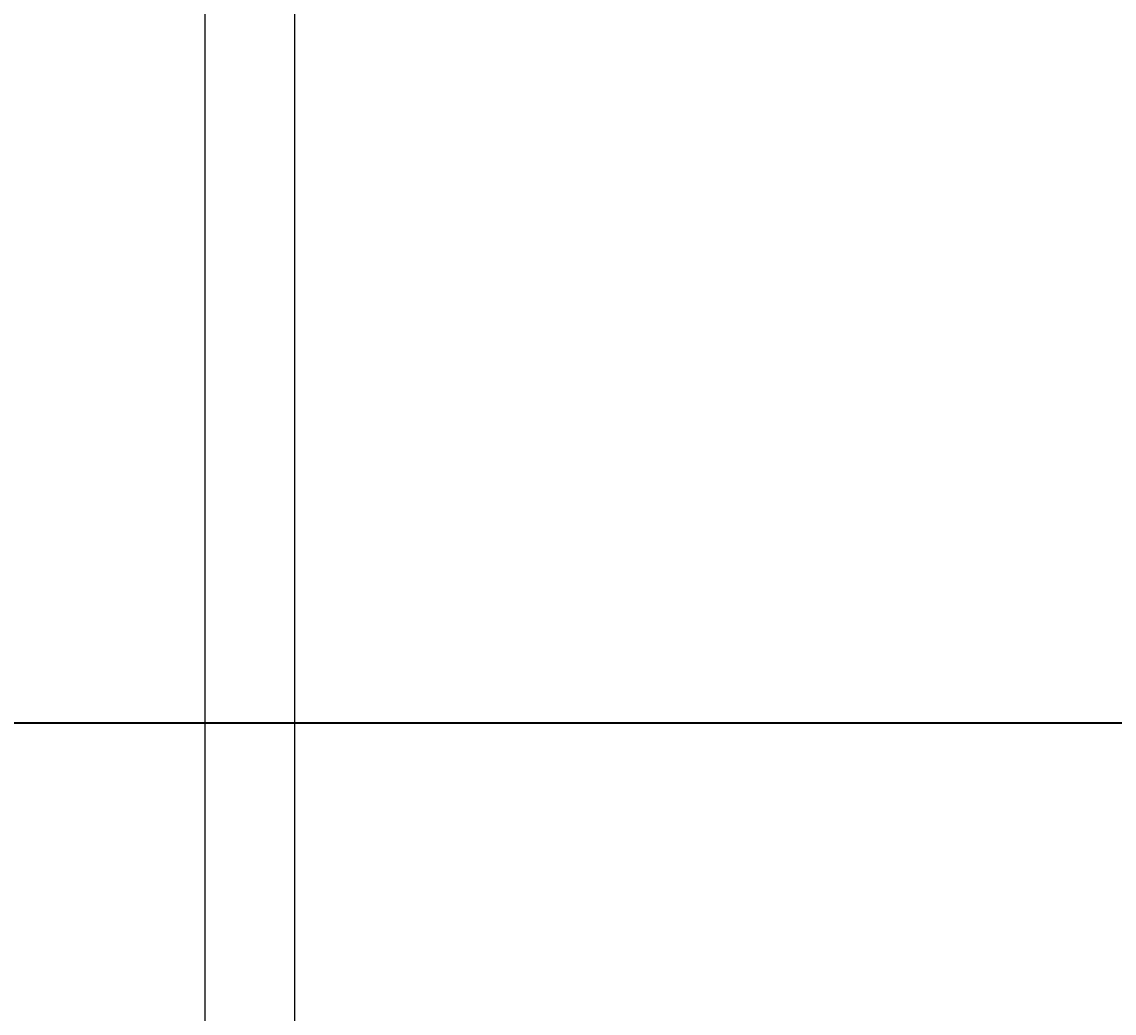
# Model space of a CAD drawing. Units: inches. Extents: x -6 to 289, y -8 to 323.
# Tile 94 of 107: x 196 to 222, y 252 to 276. Entities that reach past the tile are written whole.
import ezdxf

# ---------------------------------------------------------------- set-up
doc = ezdxf.new("R2010")
doc.units = ezdxf.units.IN
doc.header["$MEASUREMENT"] = 0
doc.layers.add('A-ANNO-DIMS', color=2, linetype='Continuous', lineweight=18)
doc.layers.add('A-ELEV', color=7, linetype='Continuous', lineweight=35)
doc.styles.get("Standard").update_dxf_attribs({"font": 'arial.ttf'})
doc.dimstyles.get("Standard").update_dxf_attribs({"dimtxt": 0.18, "dimasz": 0.18, "dimexe": 0.18, "dimexo": 0.0625, "dimgap": 0.09, "dimtad": 0, "dimtih": 1, "dimtoh": 1, "dimdec": 4, "dimzin": 0, "dimdsep": 46, "dimtxsty": 'Standard', "dimcen": 0.09, "dimadec": 0, "dimazin": 0, "dimtfac": 1, "dimtdec": 4, "dimtofl": 0, "dimtmove": 0, "dimatfit": 3, "dimfxl": 1, "dimtolj": 1, "dimtzin": 0, "dimarcsym": 0})

# ---------------------------------------------------------------- blocks, each defined once
blk = doc.blocks.new('*D13')
at = {"layer": 'A-ANNO-DIMS', "color": 0, "lineweight": -2, "transparency": 16777216}
for p, q in [((188.292, 226.951), (188.292, 322.969)), ((236.292, 226.951), (236.292, 322.969)), ((188.472, 322.789), (212.069, 322.789)), ((236.112, 322.789), (212.515, 322.789))]:
    blk.add_line(p, q, dxfattribs=at)
at = {"layer": 'A-ANNO-DIMS', "color": 0, "transparency": 16777216}
for points in [[(188.472, 322.819), (188.472, 322.759), (188.292, 322.789)], [(236.112, 322.819), (236.112, 322.759), (236.292, 322.789)]]:
    blk.add_solid(points, dxfattribs=at)
at = {"layer": 'Defpoints', "color": 0, "transparency": 16777216}
for p in [(236.292, 322.789), (188.292, 226.889), (236.292, 226.889)]:
    blk.add_point(p, dxfattribs=at)
at = {"layer": 'A-ANNO-DIMS', "color": 0, "transparency": 16777216, "insert": (212.292, 322.789), "char_height": 0.18, "attachment_point": 5}
blk.add_mtext('\\A1;48', dxfattribs=at)
blk = doc.blocks.new('*D27')
at = {"layer": 'A-ANNO-DIMS', "color": 0, "lineweight": -2, "transparency": 16777216}
for p, q in [((19.226, 307.289), (288.653, 307.289)), ((288.473, 307.109), (288.473, 277.471)), ((288.473, 247.469), (288.473, 277.107)), ((247.226, 247.289), (288.653, 247.289))]:
    blk.add_line(p, q, dxfattribs=at)
at = {"layer": 'A-ANNO-DIMS', "color": 0, "transparency": 16777216}
for points in [[(288.443, 307.109), (288.503, 307.109), (288.473, 307.289)], [(288.443, 247.469), (288.503, 247.469), (288.473, 247.289)]]:
    blk.add_solid(points, dxfattribs=at)
at = {"layer": 'Defpoints', "color": 0, "transparency": 16777216}
for p in [(19.164, 307.289), (288.473, 307.289), (247.164, 247.289)]:
    blk.add_point(p, dxfattribs=at)
at = {"layer": 'A-ANNO-DIMS', "color": 0, "transparency": 16777216, "insert": (288.473, 277.289), "char_height": 0.18, "attachment_point": 5}
blk.add_mtext('\\A1;60', dxfattribs=at)
blk = doc.blocks.new('*D80')
at = {"layer": 'A-ANNO-DIMS', "color": 0, "lineweight": -2, "transparency": 16777216}
for p, q in [((188.292, 116.842), (188.292, 322.969)), ((230.292, 116.842), (230.292, 322.969)), ((188.472, 322.789), (209.07, 322.789)), ((230.112, 322.789), (209.513, 322.789))]:
    blk.add_line(p, q, dxfattribs=at)
at = {"layer": 'A-ANNO-DIMS', "color": 0, "transparency": 16777216}
for points in [[(188.472, 322.819), (188.472, 322.759), (188.292, 322.789)], [(230.112, 322.819), (230.112, 322.759), (230.292, 322.789)]]:
    blk.add_solid(points, dxfattribs=at)
at = {"layer": 'Defpoints', "color": 0, "transparency": 16777216}
for p in [(230.292, 322.789), (188.292, 116.779), (230.292, 116.779)]:
    blk.add_point(p, dxfattribs=at)
at = {"layer": 'A-ANNO-DIMS', "color": 0, "transparency": 16777216, "insert": (209.292, 322.789), "char_height": 0.18, "attachment_point": 5}
blk.add_mtext('\\A1;42', dxfattribs=at)
blk = doc.blocks.new('*D96')
at = {"layer": 'A-ANNO-DIMS', "color": 0, "lineweight": -2, "transparency": 16777216}
for p, q in [((164.004, 159.411), (164.004, 322.969)), ((200.616, 159.411), (200.616, 322.969)), ((164.184, 322.789), (181.934, 322.789)), ((200.436, 322.789), (182.686, 322.789))]:
    blk.add_line(p, q, dxfattribs=at)
at = {"layer": 'A-ANNO-DIMS', "color": 0, "transparency": 16777216}
for points in [[(164.184, 322.819), (164.184, 322.759), (164.004, 322.789)], [(200.436, 322.819), (200.436, 322.759), (200.616, 322.789)]]:
    blk.add_solid(points, dxfattribs=at)
at = {"layer": 'Defpoints', "color": 0, "transparency": 16777216}
for p in [(200.616, 322.789), (164.004, 159.348), (200.616, 159.348)]:
    blk.add_point(p, dxfattribs=at)
at = {"layer": 'A-ANNO-DIMS', "color": 0, "transparency": 16777216, "insert": (182.31, 322.789), "char_height": 0.18, "attachment_point": 5}
blk.add_mtext('\\A1;36.61', dxfattribs=at)
blk = doc.blocks.new('*D97')
at = {"layer": 'A-ANNO-DIMS', "color": 0, "lineweight": -2, "transparency": 16777216}
for p, q in [((200.616, 159.411), (200.616, 322.969)), ((202.741, 159.411), (202.741, 322.969)), ((200.796, 322.789), (201.283, 322.789)), ((202.561, 322.789), (202.075, 322.789))]:
    blk.add_line(p, q, dxfattribs=at)
at = {"layer": 'A-ANNO-DIMS', "color": 0, "transparency": 16777216}
for points in [[(200.796, 322.819), (200.796, 322.759), (200.616, 322.789)], [(202.561, 322.819), (202.561, 322.759), (202.741, 322.789)]]:
    blk.add_solid(points, dxfattribs=at)
at = {"layer": 'Defpoints', "color": 0, "transparency": 16777216}
for p in [(202.741, 322.789), (200.616, 159.348), (202.741, 159.348)]:
    blk.add_point(p, dxfattribs=at)
at = {"layer": 'A-ANNO-DIMS', "color": 0, "transparency": 16777216, "insert": (201.679, 322.789), "char_height": 0.18, "attachment_point": 5}
blk.add_mtext('\\A1;2.125', dxfattribs=at)
blk = doc.blocks.new('*D98')
at = {"layer": 'A-ANNO-DIMS', "color": 0, "lineweight": -2, "transparency": 16777216}
for p, q in [((202.741, 159.411), (202.741, 322.969)), ((244.164, 159.411), (244.164, 322.969)), ((202.921, 322.789), (223.056, 322.789)), ((243.984, 322.789), (223.849, 322.789))]:
    blk.add_line(p, q, dxfattribs=at)
at = {"layer": 'A-ANNO-DIMS', "color": 0, "transparency": 16777216}
for points in [[(202.921, 322.819), (202.921, 322.759), (202.741, 322.789)], [(243.984, 322.819), (243.984, 322.759), (244.164, 322.789)]]:
    blk.add_solid(points, dxfattribs=at)
at = {"layer": 'Defpoints', "color": 0, "transparency": 16777216}
for p in [(244.164, 322.789), (202.741, 159.348), (244.164, 159.348)]:
    blk.add_point(p, dxfattribs=at)
at = {"layer": 'A-ANNO-DIMS', "color": 0, "transparency": 16777216, "insert": (223.452, 322.789), "char_height": 0.18, "attachment_point": 5}
blk.add_mtext('\\A1;41.42', dxfattribs=at)

msp = doc.modelspace()

# ---------------------------------------------------------------- linework, layer by layer
at = {"layer": 'A-ELEV'}
msp.add_line((115.1638, 259.2888), (271.1638, 259.2888), dxfattribs=at)

# ---------------------------------------------------------------- dimensions: what is measured, and where the dimension line sits
at = {"layer": 'A-ANNO-DIMS'}
for base, p1, p2, override, picture, middle in [((200.6162, 322.7888), (164.0039, 159.3484), (200.6162, 159.3484), {"dimdec": 2, "dimlfac": 1, "dimrnd": 0, "dimzin": 0, "dimdsep": 46, "dimlunit": 2}, '*D96', (182.3101, 322.7888)), ((236.2918, 322.7888), (188.2918, 226.8887), (236.2918, 226.8887), {"dimdec": 0, "dimlfac": 1, "dimrnd": 0, "dimzin": 0, "dimdsep": 46, "dimlunit": 2}, '*D13', (212.2918, 322.7888)), ((230.2918, 322.7888), (188.2918, 116.7795), (230.2918, 116.7795), {"dimdec": 0, "dimlfac": 1, "dimrnd": 0, "dimzin": 0, "dimdsep": 46, "dimlunit": 2}, '*D80', (209.2918, 322.7888)), ((202.741, 322.7888), (200.6162, 159.3484), (202.741, 159.3484), {"dimdec": 3, "dimlfac": 1, "dimrnd": 0, "dimzin": 0, "dimdsep": 46, "dimlunit": 2}, '*D97', (201.6786, 322.7888)), ((244.1638, 322.7888), (202.741, 159.3484), (244.1638, 159.3484), {"dimdec": 2, "dimlfac": 1, "dimrnd": 0, "dimzin": 0, "dimdsep": 46, "dimlunit": 2}, '*D98', (223.4524, 322.7888))]:
    dim = msp.add_linear_dim(base=base, p1=p1, p2=p2, dimstyle='Standard', override=override, dxfattribs=at)
    dim.commit()
    dim.dimension.update_dxf_attribs({"geometry": picture, "text_midpoint": middle})
dim = msp.add_linear_dim(base=(288.4733, 307.2888), p1=(247.1638, 247.2888), p2=(19.1638, 307.2888), angle=90, dimstyle='Standard', override={"dimdec": 0, "dimlfac": 1, "dimrnd": 0, "dimzin": 0, "dimdsep": 46, "dimlunit": 2}, dxfattribs=at)
dim.commit()
dim.dimension.update_dxf_attribs({"geometry": '*D27', "text_midpoint": (288.4733, 277.2888)})

doc.saveas('drawing.dxf')
